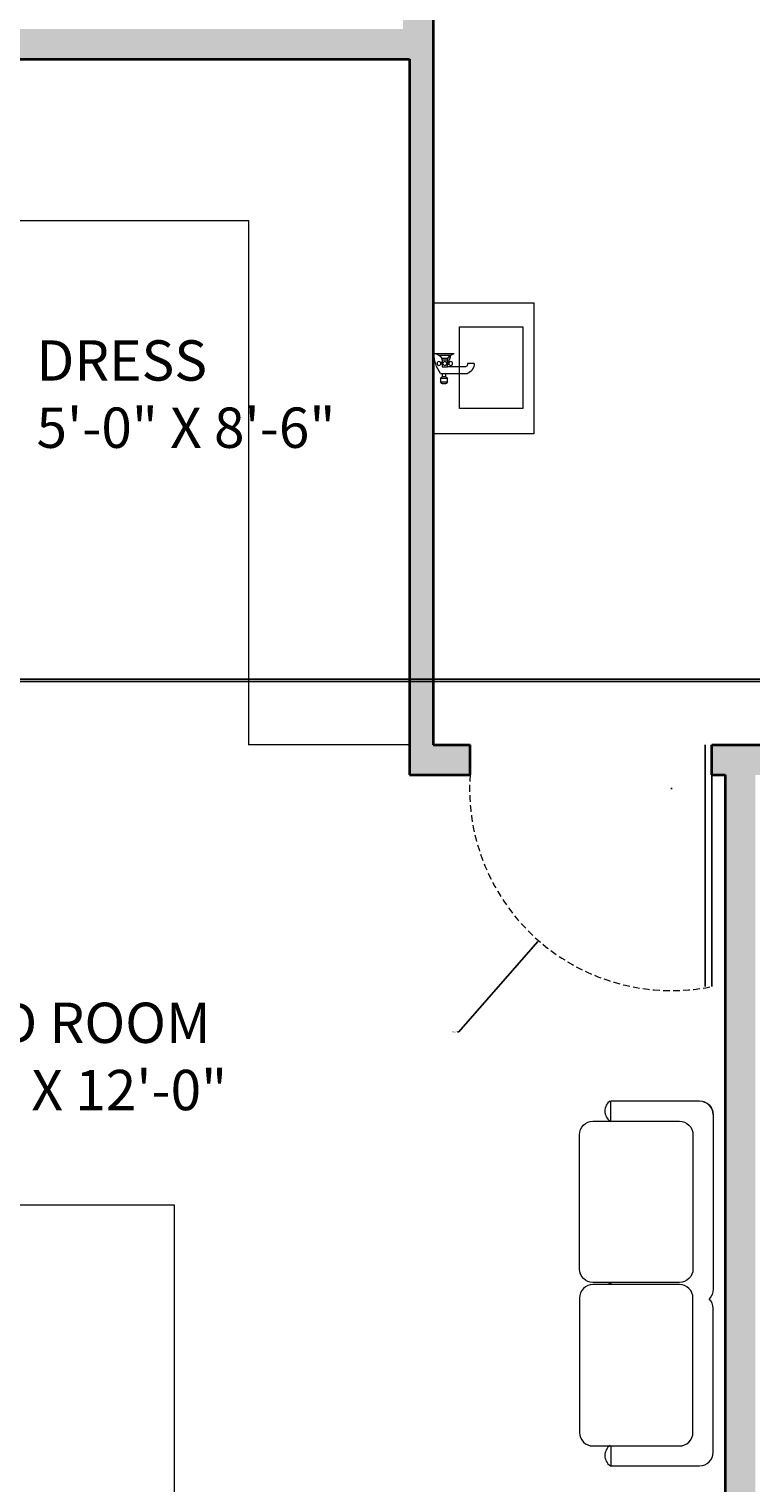
# Model space of a CAD drawing. Units: inches. Extents: x 1693 to 2974, y 2201 to 2965.
# Tile 3 of 24: x 1868 to 1976, y 2337 to 2554. Entities that reach past the tile are written whole.
import ezdxf

# ---------------------------------------------------------------- set-up
doc = ezdxf.new("R2010")
doc.units = ezdxf.units.IN
doc.header["$LTSCALE"] = 2
doc.header["$MEASUREMENT"] = 0
doc.linetypes.add('HIDDEN', pattern=[0.375, 0.25, -0.125])
for name, color, linetype, lineweight in [('A-ANNO-DIMS', 2, 'Continuous', 18), ('A-AREA-IDEN', 7, 'Continuous', 18), ('A-DOOR', 3, 'Continuous', 25), ('A-DOOR-SWNG', 3, 'HIDDEN', 13), ('A-FLOR-CASE', 32, 'Continuous', 18), ('A-FLOR-FIXT', 9, 'Continuous', 18), ('A-FURN', 8, 'Continuous', 18), ('A-WALL', 7, 'Continuous', 35)]:
    doc.layers.add(name, color=color, linetype=linetype, lineweight=lineweight)
doc.layers.add('A-WALL-PATT', color=251, linetype='Continuous', lineweight=13, true_color=0x636466)
doc.styles.get("Standard").update_dxf_attribs({"font": 'arial.ttf'})
doc.dimstyles.get("Standard").update_dxf_attribs({"dimtxt": 0.18, "dimasz": 0.18, "dimexe": 0.18, "dimexo": 0.0625, "dimgap": 0.09, "dimtad": 0, "dimtih": 1, "dimtoh": 1, "dimdec": 1, "dimzin": 0, "dimdsep": 46, "dimlunit": 3, "dimtxsty": 'Standard', "dimcen": 0.09, "dimadec": 0, "dimazin": 0, "dimtfac": 1, "dimtdec": 1, "dimtofl": 0, "dimtmove": 0, "dimatfit": 3, "dimfxl": 1, "dimtolj": 1, "dimtzin": 0, "dimarcsym": 0})

# ---------------------------------------------------------------- blocks, each defined once
blk = doc.blocks.new('Faucet - Bathroom side')
for p, q in [((-0.625, 4.25), (0.375, 4.25)), ((0.375, 3.75), (-0.625, 3.75)), ((-0.625, 3), (3.375, 3)), ((-0.375, 3), (-0.375, 3.5)), ((0.125, 3.5), (0.125, 3)), ((-1.625, 0), (-1.375, 0)), ((-1.375, 0), (1.375, 0)), ((-0.88366, 0.25), (0.88424, 0.25)), ((-0.375, 1.625), (-0.625, 1.625)), ((-0.375, 1.375), (-0.625, 1.375)), ((0.48078, 0.75), (-0.47286, 0.75)), ((2.875, 2), (0.375, 2)), ((0.375, 1.625), (0.625, 1.625)), ((0.375, 1.375), (0.625, 1.375)), ((4.375, 1.5), (3.375, 1.5))]:
    blk.add_line(p, q)
for points in [[(-0.375, 4.5), (0.125, 4.5)], [(-0.625, 3.75), (-0.625, 4.25)], [(0.125, 3.5), (-0.375, 3.5)], [(0.375, 4.25), (0.375, 3.75)]]:
    blk.add_lwpolyline(points)
blk.add_lwpolyline([(-0.375, 1), (-0.375, 2), (0.375, 2), (0.375, 1)], close=True)
for centre in [(-0.875, 1.5), (0, 1.5), (0.875, 1.5)]:
    blk.add_circle(centre, 0.27951)
for centre, radius, start, end in [((-0.38253, 4.2575), 0.24259, 88.22243, 181.7776), ((0.13252, 4.2575), 0.24259, 358.2224, 91.77757), ((3.45929, -0.0281), 5.08436, 143.4467, 179.6834), ((-0.38253, 3.7424), 0.24259, 178.2224, 271.7776), ((0.13252, 3.7424), 0.24259, 268.2224, 1.777565), ((2.70708, 1.4714), 1.66816, 0.9827695, 66.39737), ((-1.75, 1.375), 1.42522, 285.2551, 344.7449), ((1.75, 1.375), 1.42522, 195.2551, 254.7449), ((-2.49562, -0.286), 3.38273, 9.709485, 29.48735), ((2.96867, 1.5936), 0.41699, 347.0192, 102.9808)]:
    blk.add_arc(centre, radius, start, end)
blk = doc.blocks.new('Bed - Queen')
for p, q in [((0, -80.00003), (0, 0)), ((0, 0), (59.99999, 0)), ((59.99999, 0), (59.99999, -80.00003)), ((7.99999, -1.2), (28.79998, -1.2)), ((7.99999, -14.4), (7.99999, -1.2)), ((28.79998, -1.2), (28.79998, -14.4)), ((31.19999, -1.2), (51.99999, -1.2)), ((31.19999, -14.4), (31.19999, -1.2)), ((51.99999, -1.2), (51.99999, -16.4)), ((0, -14.4), (44.8, -14.4)), ((59.99999, -29.6), (44.8, -14.4)), ((44.8, -14.4), (44.8, -29.6)), ((44.8, -16.8), (0, -16.8)), ((51.99999, -16.4), (46.79936, -16.4)), ((44.8, -29.6), (59.99999, -29.6)), ((59.99999, -80.00003), (0, -80.00003))]:
    blk.add_line(p, q)
blk = doc.blocks.new('SOFA-2-SEAT')
at = {"ltscale": 2}
for p, q in [((17.9, 54.27), (4.68, 54.27)), ((4.68, 51.27), (4.68, 54.27)), ((4.68, 51.27), (4.68, 51.55)), ((4.68, 27.26), (4.68, 26.96)), ((19.9, 2), (19.9, 23.43)), ((4.68, 3), (4.68, 0)), ((4.59, 0), (17.9, 0))]:
    blk.add_line(p, q, dxfattribs=at)
for points in [[(18.47, 54.18, -0.331344), (19.9, 52.27), (19.9, 26.26, -0.198912), (19.31, 24.85)], [(0, 49.27, -0.414214), (2, 51.27), (14.9, 51.27, -0.414214), (16.9, 49.27), (16.9, 29.26, -0.414214), (14.9, 27.26), (2, 27.26, -0.414214), (0, 29.26), (0, 49.27)], [(0, 4.95, 0.414214), (2, 2.95), (14.9, 2.95, 0.414214), (16.9, 4.95), (16.9, 24.96, 0.414214), (14.9, 26.96), (2, 26.96, 0.414214), (0, 24.96), (0, 4.95)]]:
    blk.add_lwpolyline(points, format="xyb", dxfattribs=at)
for centre, radius, start, end in [((5.65, 52.79), 1.86, 125.0084, 234.9916), ((17.9, 52.27), 2, 0, 90), ((5.65, 52.75), 1.86, 219.881, 234.9916), ((5.65, 25.74), 1.86, 125.0084, 139.1343), ((17.9, 23.43), 2, 0, 45), ((5.65, 1.52), 1.86, 125.0084, 234.9916), ((17.9, 2), 2, 270, 0)]:
    blk.add_arc(centre, radius, start, end, dxfattribs=at)
blk = doc.blocks.new('BASIN-WALL-MOUNT')
at = {"ltscale": 2}
for points in [[(15.01, 19.49), (0, 19.49), (0, 0), (15.01, 0)], [(11.1, 15.94), (1.63, 15.94), (1.63, 3.76), (11.1, 3.76)]]:
    blk.add_lwpolyline(points, close=True, dxfattribs=at)
blk = doc.blocks.new('*D81')
at = {"layer": 'A-ANNO-DIMS', "color": 0, "lineweight": -2, "ltscale": 2, "transparency": 16777216}
for p, q in [((1752.34, 2553.91), (1752.34, 2964.96)), ((1752.52, 2964.78), (2332.94, 2964.78)), ((2914.06, 2964.78), (2333.64, 2964.78)), ((2914.24, 2754.97), (2914.24, 2964.96))]:
    blk.add_line(p, q, dxfattribs=at)
at = {"layer": 'A-ANNO-DIMS', "color": 0, "ltscale": 2, "transparency": 16777216}
for points in [[(1752.52, 2964.81), (1752.52, 2964.75), (1752.34, 2964.78)], [(2914.06, 2964.81), (2914.06, 2964.75), (2914.24, 2964.78)]]:
    blk.add_solid(points, dxfattribs=at)
at = {"layer": 'Defpoints', "color": 0, "ltscale": 2, "transparency": 16777216}
for p in [(2914.24, 2964.78), (2914.24, 2754.9), (1752.34, 2553.84)]:
    blk.add_point(p, dxfattribs=at)
at = {"layer": 'A-ANNO-DIMS', "color": 0, "ltscale": 2, "transparency": 16777216, "insert": (2333.29, 2964.78), "char_height": 0.18, "attachment_point": 5}
blk.add_mtext('\\A1;1162', dxfattribs=at)
blk = doc.blocks.new('*D82')
at = {"layer": 'A-ANNO-DIMS', "color": 0, "lineweight": -2, "ltscale": 2, "transparency": 16777216}
for p, q in [((2615.67, 2906.08), (1693.46, 2906.08)), ((1693.64, 2905.9), (1693.64, 2582.94)), ((1693.64, 2259.62), (1693.64, 2582.58)), ((2096.17, 2259.44), (1693.46, 2259.44))]:
    blk.add_line(p, q, dxfattribs=at)
at = {"layer": 'A-ANNO-DIMS', "color": 0, "ltscale": 2, "transparency": 16777216}
for points in [[(1693.61, 2905.9), (1693.67, 2905.9), (1693.64, 2906.08)], [(1693.61, 2259.62), (1693.67, 2259.62), (1693.64, 2259.44)]]:
    blk.add_solid(points, dxfattribs=at)
at = {"layer": 'Defpoints', "color": 0, "ltscale": 2, "transparency": 16777216}
for p in [(1693.64, 2906.08), (2615.74, 2906.08), (2096.24, 2259.44)]:
    blk.add_point(p, dxfattribs=at)
at = {"layer": 'A-ANNO-DIMS', "color": 0, "ltscale": 2, "transparency": 16777216, "insert": (1693.64, 2582.76), "char_height": 0.18, "attachment_point": 5}
blk.add_mtext('\\A1;646.6', dxfattribs=at)
blk = doc.blocks.new('*D108')
at = {"layer": 'A-ANNO-DIMS', "color": 0, "lineweight": -2, "ltscale": 2, "transparency": 16777216}
for p, q in [((1752.74, 2457.09), (2973.12, 2457.09)), ((1752.74, 2456.73), (2973.12, 2456.73)), ((2972.94, 2457.27), (2972.94, 2457.45)), ((2972.94, 2457.45), (2973.12, 2457.45)), ((2972.94, 2456.55), (2972.94, 2456.37))]:
    blk.add_line(p, q, dxfattribs=at)
at = {"layer": 'A-ANNO-DIMS', "color": 0, "ltscale": 2, "transparency": 16777216}
for points in [[(2972.91, 2457.27), (2972.97, 2457.27), (2972.94, 2457.09)], [(2972.91, 2456.55), (2972.97, 2456.55), (2972.94, 2456.73)]]:
    blk.add_solid(points, dxfattribs=at)
at = {"layer": 'Defpoints', "color": 0, "ltscale": 2, "transparency": 16777216}
for p in [(1752.68, 2457.09), (1752.68, 2456.73), (2972.94, 2457.09)]:
    blk.add_point(p, dxfattribs=at)
at = {"layer": 'A-ANNO-DIMS', "color": 0, "ltscale": 2, "transparency": 16777216, "insert": (2973.44, 2457.45), "char_height": 0.18, "attachment_point": 5}
blk.add_mtext('\\A1;0.36', dxfattribs=at)
blk = doc.blocks.new('*D120')
at = {"layer": 'A-ANNO-DIMS', "color": 0, "lineweight": -2, "ltscale": 2, "transparency": 16777216}
for p, q in [((1963.67, 2440.83), (1963.85, 2440.83)), ((1963.76, 2440.74), (1963.76, 2440.92)), ((1932.06, 2404.6), (1943.83, 2418.05)), ((1931.88, 2404.6), (1932.06, 2404.6))]:
    blk.add_line(p, q, dxfattribs=at)
at = {"layer": 'A-ANNO-DIMS', "color": 0, "ltscale": 2, "transparency": 16777216}
blk.add_solid([(1943.8, 2418.07), (1943.85, 2418.03), (1943.94, 2418.19)], dxfattribs=at)
at = {"layer": 'Defpoints', "color": 0, "ltscale": 2, "transparency": 16777216}
for p in [(1963.76, 2440.83), (1943.94, 2418.19)]:
    blk.add_point(p, dxfattribs=at)
at = {"layer": 'A-ANNO-DIMS', "color": 0, "ltscale": 2, "transparency": 16777216, "insert": (1931.4, 2404.6), "char_height": 0.18, "attachment_point": 5}
blk.add_mtext('\\A1;R30.09', dxfattribs=at)

msp = doc.modelspace()

# ---------------------------------------------------------------- hatches: boundary and pattern name
at = {"layer": 'A-WALL-PATT', "ltscale": 2}
h = msp.add_hatch(color=256, dxfattribs=at)
h.dxf.hatch_style = 1
h.paths.add_polyline_path([(1928.2363, 2733.2161), (1930.9384, 2733.2161), (1930.9384, 2737.2161), (1923.7363, 2737.2161), (1923.7363, 2706.8449), (1908.1286, 2706.8449), (1908.1286, 2697.8449), (1923.7363, 2697.8449), (1923.7363, 2692.8449), (1928.2363, 2692.8449), (1928.2363, 2697.8449), (1949.9863, 2697.8449), (1949.9863, 2706.8449), (1928.2363, 2706.8449)])
h.paths.add_polyline_path([(2004.7363, 2737.2161), (1995.7363, 2737.2161), (1995.7363, 2706.8449), (1985.6374, 2706.8449), (1973.9863, 2706.8449), (1973.9863, 2697.8449), (2000.2363, 2697.8449), (2000.2363, 2686.5348), (2000.3613, 2686.5348), (2000.3613, 2667.0432), (2000.2363, 2601.8449), (1928.2363, 2601.8449), (1928.2363, 2662.8449), (1923.7363, 2662.8449), (1923.7363, 2595.3449), (1928.2363, 2595.3449), (1928.2363, 2597.3449), (2004.7363, 2597.3449), (2004.7363, 2681.3449), (2012.7814, 2681.3449), (2028.7363, 2681.3449), (2028.7363, 2690.3449), (2004.7363, 2690.3449)])
h.paths.add_polyline_path([(2190.9863, 2706.8449), (2184.9863, 2706.8449), (2145.7363, 2706.8449), (2145.7363, 2765.3449), (2145.7363, 2774.5394), (2136.7363, 2774.5394), (2136.7363, 2756.3449), (2136.7363, 2690.3449), (2112.7363, 2690.3449), (2112.7363, 2681.3449), (2136.7363, 2681.3449), (2136.7363, 2597.3449), (2141.2363, 2597.3449), (2141.2363, 2697.8449), (2190.9863, 2697.8449)])
h.paths.add_polyline_path([(1860.1286, 2706.8449), (1782.7363, 2706.8449), (1782.7363, 2621.6433), (1791.7363, 2621.6433), (1791.7363, 2697.8449), (1860.1286, 2697.8449)])
h.paths.add_polyline_path([(1791.7363, 2585.6433), (1782.7363, 2585.6433), (1782.7363, 2562.8449), (1782.7363, 2553.8449), (1752.3363, 2553.8449), (1752.3363, 2544.2586), (1756.3363, 2544.2586), (1756.3363, 2549.3449), (1782.7363, 2549.3449), (1782.7363, 2489.2404), (1782.7363, 2477.5455), (1791.7363, 2477.5455), (1791.7363, 2493.5991), (1791.6113, 2493.5991), (1791.6113, 2513.0907), (1791.6824, 2533.7198, -0.94742783), (1791.7363, 2534.7168), (1791.7363, 2549.3449), (1863.7363, 2549.3449), (1863.7363, 2513.3449), (1866.7363, 2513.3449), (1866.7363, 2549.3449), (1924.7363, 2549.3449), (1924.7363, 2447.3449), (1924.7363, 2442.8449), (1933.7363, 2442.8449), (1933.7363, 2447.3449), (1928.2363, 2447.3449), (1928.2363, 2559.3449), (1923.7363, 2559.3449), (1923.7363, 2553.8449), (1791.7363, 2553.8449), (1791.7363, 2562.8449)])
h.paths.add_polyline_path([(1791.7363, 2442.8449), (1866.7363, 2442.8449), (1866.7363, 2447.3449), (1866.7363, 2483.3449), (1863.7363, 2483.3449), (1863.7363, 2447.3449), (1791.7363, 2447.3449), (1791.7363, 2453.5455), (1782.7363, 2453.5455), (1782.7363, 2447.3449), (1756.3363, 2447.3449), (1756.3363, 2455.7126), (1752.3363, 2455.7126), (1752.3363, 2442.8449), (1782.7363, 2442.8449), (1782.7363, 2403.1922), (1791.7363, 2403.1922)])
h.paths.add_polyline_path([(1930.0781, 2298.8449), (1791.7363, 2298.8449), (1791.7363, 2355.1922), (1782.7363, 2355.1922), (1782.7363, 2289.8449), (1930.0781, 2289.8449)])
h.paths.add_polyline_path([(2624.7363, 2883.2547), (2624.7363, 2902.6165), (2624.7363, 2906.0761), (2615.7363, 2906.0761), (2615.7363, 2892.2547), (2615.7363, 2846.2547), (2578.2363, 2846.2547), (2578.2363, 2837.2547), (2620.2363, 2837.2547), (2620.2363, 2743.2547), (2624.7363, 2743.2547), (2624.7363, 2808.2547), (2648.7363, 2808.2547), (2648.7363, 2817.2547), (2624.7363, 2817.2547)])
h.paths.add_polyline_path([(2530.2363, 2846.2547), (2479.2363, 2846.2547), (2479.2363, 2695.8203), (2488.2363, 2695.8203), (2488.2363, 2700.7547), (2567.2363, 2700.7547), (2567.2363, 2705.2547), (2488.2363, 2705.2547), (2488.2363, 2837.2547), (2530.2363, 2837.2547)])
h.paths.add_polyline_path([(2488.2363, 2487.7547), (2630.2363, 2487.7547, -0.00990191), (2630.2363, 2489.0322), (2630.2363, 2492.2547), (2488.2363, 2492.2547), (2488.2363, 2512.4371), (2479.2363, 2512.4371), (2479.2363, 2334.7547), (2608.9702, 2334.7547), (2608.9702, 2343.7547), (2488.2363, 2343.7547)])
h.paths.add_polyline_path([(2751.7544, 2343.7547), (2672.7363, 2343.7547), (2672.7363, 2409.7547), (2674.7363, 2409.7547), (2674.7363, 2413.7547), (2672.7363, 2413.7547), (2672.7363, 2487.7547), (2732.7363, 2487.7547), (2732.7363, 2413.7547), (2704.7363, 2413.7547), (2704.7363, 2409.7547), (2784.7363, 2409.7547), (2784.7363, 2343.7547), (2775.7544, 2343.7547), (2775.7544, 2334.7547), (2902.2363, 2334.7547), (2902.2363, 2520.7999), (2893.2363, 2520.7999), (2893.2363, 2413.7547), (2856.0145, 2413.7547), (2856.0145, 2409.7547), (2893.2363, 2409.7547), (2893.2363, 2343.7547), (2789.2363, 2343.7547), (2789.2363, 2409.7547), (2819.2363, 2409.7547), (2826.0145, 2409.7547), (2826.0145, 2413.7547), (2789.2363, 2413.7547), (2789.2363, 2492.2547), (2784.7363, 2492.2547), (2784.7363, 2413.7547), (2736.7363, 2413.7547), (2736.7363, 2492.2547), (2672.7363, 2492.2547), (2666.2363, 2492.2547), (2666.2363, 2487.7547), (2668.2363, 2487.7547), (2668.2363, 2343.7547), (2656.9702, 2343.7547), (2656.9702, 2334.7547), (2662.9702, 2334.7547), (2751.7544, 2334.7547)])
h.paths.add_polyline_path([(2902.2363, 2613.7547), (2893.2363, 2613.7547), (2893.2363, 2589.7547), (2785.2363, 2589.7547), (2785.2363, 2661.7547), (2790.2363, 2661.7547), (2790.2363, 2665.2547), (2761.2363, 2665.2547), (2761.2363, 2667.2547), (2756.7363, 2667.2547), (2756.7363, 2661.7547), (2781.2363, 2661.7547), (2781.2363, 2585.7547), (2893.2363, 2585.7547), (2893.2363, 2568.7999), (2902.2363, 2568.7999)])
h.paths.add_polyline_path([(2488.2363, 2671.8203), (2479.2363, 2671.8203), (2479.2363, 2645.2547), (2479.2363, 2623.4598), (2488.2363, 2623.4598), (2488.2363, 2636.2547), (2624.7363, 2636.2547), (2624.7363, 2640.7547), (2603.7363, 2640.7547), (2603.7363, 2700.7547), (2624.7363, 2700.7547), (2624.7363, 2707.2547), (2620.2363, 2707.2547), (2620.2363, 2705.2547), (2597.2363, 2705.2547), (2597.2363, 2700.7547), (2599.2363, 2700.7547), (2599.2363, 2640.7547), (2488.2363, 2640.7547)])
h.paths.add_polyline_path([(2761.2363, 2837.2547), (2803.2363, 2837.2547), (2803.2363, 2846.2547), (2797.2363, 2846.2547), (2765.7363, 2846.2547), (2756.7363, 2846.2547), (2756.7363, 2817.2547), (2732.7363, 2817.2547), (2732.7363, 2808.2547), (2756.7363, 2808.2547), (2756.7363, 2703.2547), (2761.2363, 2703.2547)])
h.paths.add_polyline_path([(2739.7489, 2433.1234), (2786.9181, 2433.1234), (2786.9181, 2455.5122), (2739.7489, 2455.5122)], flags=25)
h = msp.add_hatch(color=256, dxfattribs=at)
h.dxf.hatch_style = 1
h.paths.add_polyline_path([(2294.2363, 2706.8449), (2248.9863, 2706.8449), (2248.9863, 2697.8449), (2285.2363, 2697.8449), (2285.2363, 2586.2648), (2294.2363, 2586.2648)])
h.paths.add_polyline_path([(2294.2363, 2550.2648), (2285.2363, 2550.2648), (2285.2363, 2517.8449), (2141.2363, 2517.8449), (2141.2363, 2513.8449), (2285.2363, 2513.8449), (2285.2363, 2369.8449), (2253.0704, 2369.8449), (2253.0704, 2366.8449), (2285.2363, 2366.8449), (2285.2363, 2298.8449), (2165.2363, 2298.8449), (2165.2363, 2366.8449), (2165.2363, 2369.8449), (2165.2363, 2447.3449), (2160.7363, 2447.3449), (2160.7363, 2403.3449), (2100.7363, 2403.3449), (2100.7363, 2447.3449), (2094.2363, 2447.3449), (2094.2363, 2442.8449), (2096.2363, 2442.8449), (2096.2363, 2362.1344), (2100.7363, 2362.1344), (2100.7363, 2400.8449), (2160.7363, 2400.8449), (2160.7363, 2298.8449), (2151.9207, 2298.8449), (2151.9207, 2289.8449), (2184.7363, 2289.8449), (2184.7363, 2276.6449), (2189.2363, 2276.6449), (2189.2363, 2289.8449), (2294.2363, 2289.8449)])
h.paths.add_polyline_path([(2048.023, 2298.8449), (1976.2363, 2298.8449), (1976.2363, 2442.8449), (2058.2363, 2442.8449, -0.00822734), (2058.2363, 2443.9061), (2058.2363, 2447.3449), (2004.7363, 2447.3449), (1969.7363, 2447.3449), (1969.7363, 2442.8449), (1971.7363, 2442.8449), (1971.7363, 2298.8449), (1966.0781, 2298.8449), (1966.0781, 2289.8449), (2048.023, 2289.8449)])
h.paths.add_polyline_path([(2127.9207, 2298.8449), (2100.7363, 2298.8449), (2100.7363, 2332.1344), (2096.2363, 2332.1344), (2096.2363, 2298.8449), (2084.023, 2298.8449), (2084.023, 2289.8449), (2096.2363, 2289.8449), (2096.2363, 2259.4449), (2114.3201, 2259.4449), (2114.3201, 2263.4449), (2100.7363, 2263.4449), (2100.7363, 2289.8449), (2127.9207, 2289.8449)])

# ---------------------------------------------------------------- linework, layer by layer
at = {"layer": 'A-DOOR', "ltscale": 2}
for p, q in [((1968.7363, 2447.3449), (1968.7363, 2411.3449)), ((1969.7363, 2447.3449), (1969.7363, 2411.3449))]:
    msp.add_line(p, q, dxfattribs=at)
at = {"layer": 'A-DOOR-SWNG', "ltscale": 2}
msp.add_arc((1963.7563, 2440.832), 30.0874, 176.163979, 281.464171, dxfattribs=at)
at = {"layer": 'A-FLOR-CASE'}
for p, q in [((1866.7363, 2525.3449), (1900.7363, 2525.3449)), ((1900.7363, 2525.3449), (1900.7363, 2447.3449))]:
    msp.add_line(p, q, dxfattribs=at)
at = {"layer": 'A-FLOR-CASE', "ltscale": 2}
msp.add_line((1924.7363, 2447.3449), (1900.7363, 2447.3449), dxfattribs=at)
at = {"layer": 'A-WALL'}
for p, q in [((1928.2363, 2559.3449), (1928.2363, 2447.3449)), ((1866.7363, 2549.3449), (1924.7363, 2549.3449)), ((1924.7363, 2549.3449), (1924.7363, 2447.3449)), ((1928.2363, 2447.3449), (1933.7363, 2447.3449)), ((1933.7363, 2442.8449), (1933.7363, 2447.3449)), ((1969.7363, 2442.8449), (1969.7363, 2447.3449)), ((1969.7363, 2447.3449), (2058.2363, 2447.3449)), ((1924.7363, 2442.8449), (1933.7363, 2442.8449)), ((1969.7363, 2442.8449), (1971.7363, 2442.8449)), ((1971.7363, 2442.8449), (1971.7363, 2298.8449))]:
    msp.add_line(p, q, dxfattribs=at)
at = {"layer": 'A-WALL', "ltscale": 2}
msp.add_line((1924.7363, 2447.3449), (1924.7363, 2442.8449), dxfattribs=at)

# ---------------------------------------------------------------- block references
at = {"layer": 'A-FLOR-FIXT', "extrusion": (0, 0, -1), "zscale": -1}
msp.add_blockref('BASIN-WALL-MOUNT', (-1943.2496, 2493.5994), dxfattribs=at)
at = {"layer": 'A-FLOR-FIXT', "ltscale": 2, "xscale": -1, "rotation": 180}
msp.add_blockref('Faucet - Bathroom side', (1929.9863, 2505.5803), dxfattribs=at)
at = {"layer": 'A-FURN'}
msp.add_blockref('SOFA-2-SEAT', (1950.0363, 2340.0329), dxfattribs=at)
at = {"layer": 'A-FURN', "ltscale": 2, "rotation": 180}
msp.add_blockref('Bed - Queen', (1889.6709, 2298.8449), dxfattribs=at)

# ---------------------------------------------------------------- texts
at = {"layer": 'A-AREA-IDEN', "ltscale": 2, "char_height": 6, "attachment_point": 1}
for s, insert in [('DRESS\\P5\'-0" X 8\'-6"', (1869.1683, 2507.523)), ('M-BED ROOM\\P15\'-0" X 12\'-0"', (1843.9618, 2408.9535))]:
    msp.add_mtext_dynamic_manual_height_columns(s, width=108.452746, gutter_width=1, heights=[0], dxfattribs=dict(at, insert=insert))

# ---------------------------------------------------------------- dimensions: what is measured, and where the dimension line sits
at = {"layer": 'A-ANNO-DIMS', "ltscale": 2}
dim = msp.add_linear_dim(base=(2914.2363, 2964.7761), p1=(1752.3363, 2553.8449), p2=(2914.2363, 2754.903), dimstyle='Standard', override={"dimdec": 0, "dimlfac": 1, "dimrnd": 0, "dimzin": 0, "dimdsep": 46, "dimlunit": 2}, dxfattribs=at)
dim.commit()
dim.dimension.update_dxf_attribs({"geometry": '*D81', "text_midpoint": (2333.2863, 2964.7761)})
for base, p1, p2, override, picture, middle in [((1693.6363, 2906.0761), (2096.2363, 2259.4449), (2615.7363, 2906.0761), {"dimdec": 1, "dimlfac": 1, "dimrnd": 0, "dimzin": 0, "dimdsep": 46, "dimlunit": 2}, '*D82', (1693.6363, 2582.7605)), ((2972.9363, 2457.0877), (1752.6754, 2456.7302), (1752.6754, 2457.0877), {"dimdec": 2, "dimlfac": 1, "dimrnd": 0, "dimzin": 0, "dimdsep": 46, "dimlunit": 2}, '*D108', (2973.44, 2457.4477))]:
    dim = msp.add_linear_dim(base=base, p1=p1, p2=p2, angle=90, dimstyle='Standard', override=override, dxfattribs=at)
    dim.commit()
    dim.dimension.update_dxf_attribs({"geometry": picture, "text_midpoint": middle})
dim = msp.add_radius_dim(center=(1963.7563, 2440.832), mpoint=(1943.9438, 2418.1888), dimstyle='Standard', override={"dimdec": 2, "dimlfac": 1, "dimrnd": 0, "dimzin": 0, "dimdsep": 46, "dimlunit": 2}, dxfattribs=at)
dim.commit()
dim.dimension.update_dxf_attribs({"geometry": '*D120', "text_midpoint": (1931.3963, 2404.6028), "dimtype": 164})

doc.saveas('drawing.dxf')
